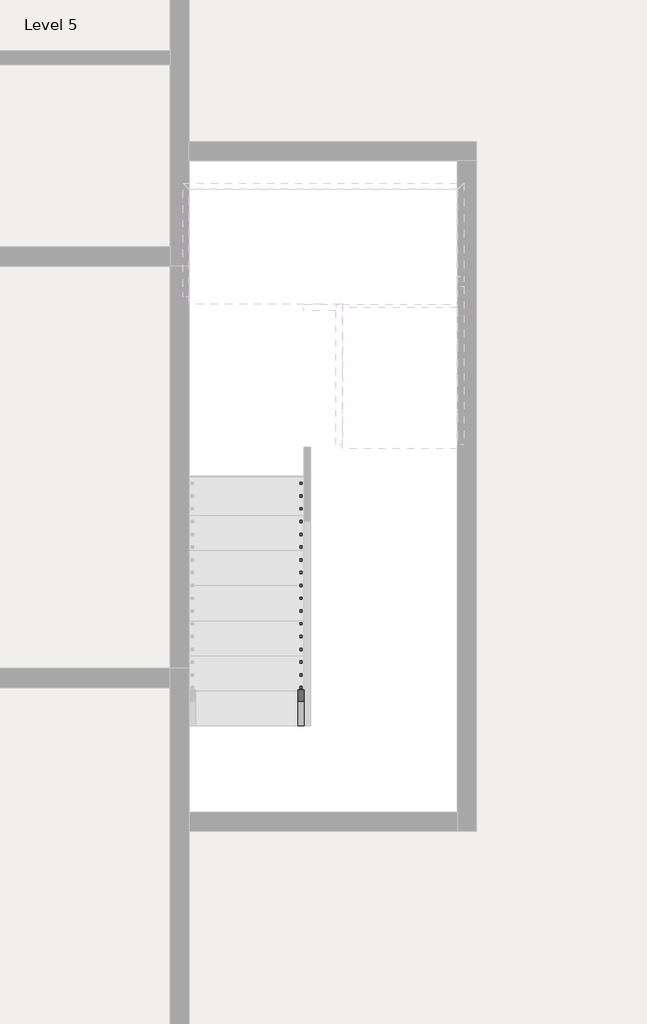
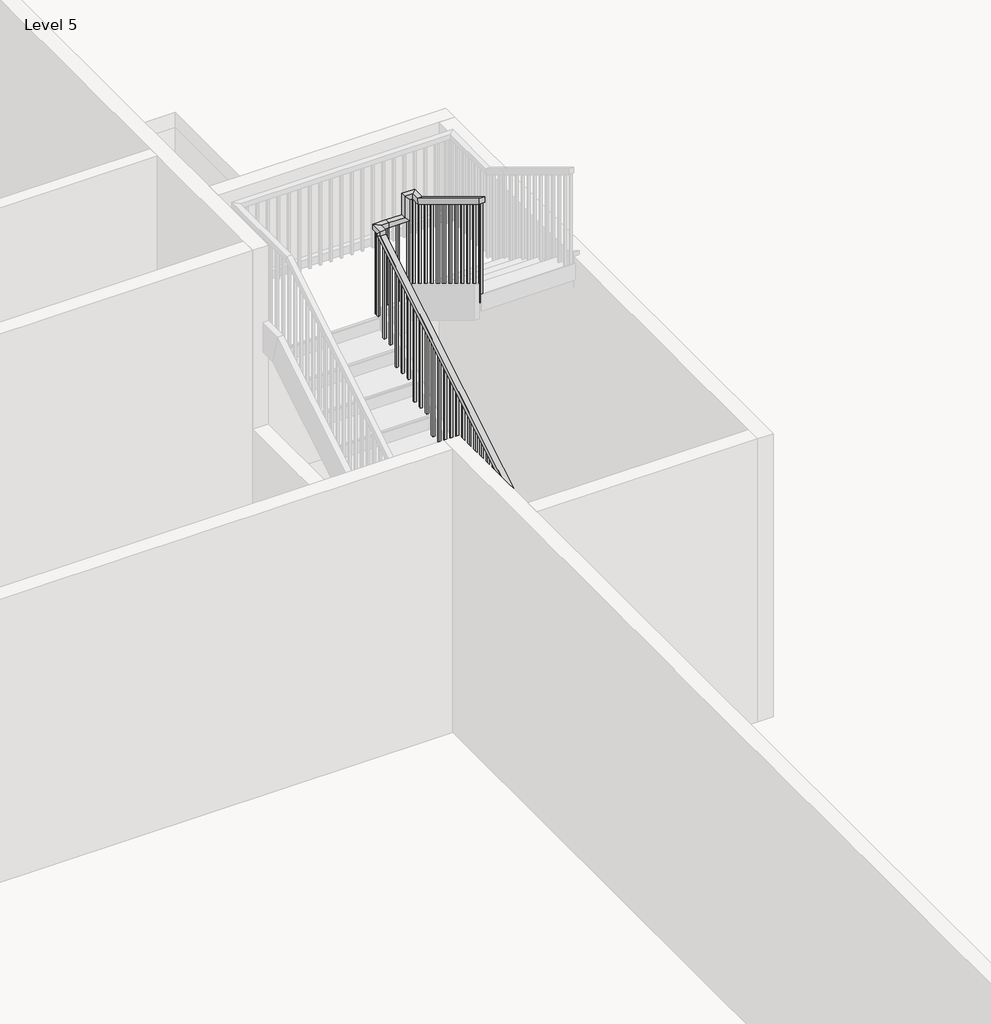
# One storey, part 7 of 8: 1 railing.
"""IFC4 building model written with IfcOpenShell, lengths in millimetres."""

from ifc_helpers import new_model, si_unit, frame, origin, place, context, project, spatial, polyline, outline, extrude, faceted_brep, element, save

model = new_model("IFC4")

# Units and contexts
model_context = context("Model", 3, world=origin())
ifc_project = project(units=[si_unit("LENGTHUNIT", "METRE", prefix="MILLI")], contexts=[model_context])

# Site, building, storey
site = spatial("IfcSite", under=ifc_project)
building = spatial("IfcBuilding", under=site)
storey = spatial("IfcBuildingStorey", under=building, Name="Level 5", Elevation=37426.6172466)

# Railing
placement = place(None, origin())
element("IfcRailing", 1, ObjectType="Handrail - Rectangular", at=placement, inside=storey, context=model_context, shape_type="SolidModel", body=[
    faceted_brep([(-2753.8415084, 19841.9216096, 38510.3505799), (-2753.8415084, 19841.9216096, 38450.9491197), (-2703.0415084, 19841.9216096, 38450.9491197), (-2703.0415084, 19841.9216096, 38510.3505799), (-2753.8415084, 23118.5216096, 40496.1687618), (-2753.8415084, 23169.3216096, 40467.5551803), (-2703.0415084, 23169.3216096, 40467.5551803), (-2703.0415084, 23118.5216096, 40496.1687618), (-2753.8415084, 23118.5216096, 40542.3505799), (-2753.8415084, 23169.3216096, 40491.5505799), (-2703.0415084, 23169.3216096, 40491.5505799), (-2703.0415084, 23118.5216096, 40542.3505799), (-2753.8415084, 23245.5216096, 40542.3505799), (-2753.8415084, 23245.5216096, 40491.5505799), (-2703.0415084, 23194.7216096, 40491.5505799), (-2703.0415084, 23194.7216096, 40542.3505799), (-2626.8415084, 23245.5216096, 40542.3505799), (-2626.8415084, 23245.5216096, 40491.5505799), (-2626.8415084, 23194.7216096, 40491.5505799), (-2626.8415084, 23194.7216096, 40542.3505799), (-2474.4415084, 23245.5216096, 40542.3505799), (-2423.6415084, 23245.5216096, 40491.5505799), (-2423.6415084, 23194.7216096, 40491.5505799), (-2474.4415084, 23194.7216096, 40542.3505799), (-2474.4415084, 23245.5216096, 40757.8657314), (-2423.6415084, 23245.5216096, 40707.0657314), (-2423.6415084, 23194.7216096, 40707.0657314), (-2474.4415084, 23194.7216096, 40757.8657314), (-2347.4415084, 23245.5216096, 40757.8657314), (-2347.4415084, 23245.5216096, 40707.0657314), (-2398.2415084, 23194.7216096, 40707.0657314), (-2398.2415084, 23194.7216096, 40757.8657314), (-2347.4415084, 23118.5216096, 40757.8657314), (-2347.4415084, 23104.3292002, 40707.0657314), (-2398.2415084, 23104.3292002, 40707.0657314), (-2398.2415084, 23118.5216096, 40757.8657314), (-2347.4415084, 22077.1216096, 41389.0172466), (-2398.2415084, 22077.1216096, 41389.0172466), (-2398.2415084, 22077.1216096, 41329.6157863), (-2347.4415084, 22077.1216096, 41329.6157863)], [[[0, 1, 2, 3]], [[1, 0, 4, 5]], [[2, 1, 5, 6]], [[3, 2, 6, 7]], [[0, 3, 7, 4]], [[5, 4, 8, 9]], [[6, 5, 9, 10]], [[7, 6, 10, 11]], [[4, 7, 11, 8]], [[9, 8, 12, 13]], [[10, 9, 13, 14]], [[11, 10, 14, 15]], [[8, 11, 15, 12]], [[13, 12, 16, 17]], [[14, 13, 17, 18]], [[15, 14, 18, 19]], [[12, 15, 19, 16]], [[17, 16, 20, 21]], [[18, 17, 21, 22]], [[19, 18, 22, 23]], [[16, 19, 23, 20]], [[21, 20, 24, 25]], [[22, 21, 25, 26]], [[23, 22, 26, 27]], [[20, 23, 27, 24]], [[25, 24, 28, 29]], [[26, 25, 29, 30]], [[27, 26, 30, 31]], [[24, 27, 31, 28]], [[29, 28, 32, 33]], [[30, 29, 33, 34]], [[31, 30, 34, 35]], [[28, 31, 35, 32]], [[36, 37, 38, 39]], [[33, 32, 36, 39]], [[34, 33, 39, 38]], [[35, 34, 38, 37]], [[32, 35, 37, 36]]]),
    extrude(outline(polyline([(22092.9966096, 41319.9945742), (22112.0466096, 41308.4491197), (22112.0466096, 40305.2839133), (22092.9966096, 40305.2839133), (22092.9966096, 41319.9945742)])), frame((-2382.3665084, 0.0, 0.0), z_axis=(1.0, 0.0, 0.0), x_axis=(0.0, 1.0, 0.0)), (0.0, 0.0, 1.0), 19.05),
    extrude(outline(polyline([(22194.5966096, 41258.4188166), (22213.6466096, 41246.8733621), (22213.6466096, 40305.2839133), (22194.5966096, 40305.2839133), (22194.5966096, 41258.4188166)])), frame((-2382.3665084, 0.0, 0.0), z_axis=(1.0, 0.0, 0.0), x_axis=(0.0, 1.0, 0.0)), (0.0, 0.0, 1.0), 19.05),
    extrude(outline(polyline([(22296.1966096, 41196.8430591), (22315.2466096, 41185.2976045), (22315.2466096, 40305.2839133), (22296.1966096, 40305.2839133), (22296.1966096, 41196.8430591)])), frame((-2382.3665084, 0.0, 0.0), z_axis=(1.0, 0.0, 0.0), x_axis=(0.0, 1.0, 0.0)), (0.0, 0.0, 1.0), 19.05),
    extrude(outline(polyline([(22397.7966096, 41135.2673015), (22416.8466096, 41123.721847), (22416.8466096, 40135.9505799), (22397.7966096, 40135.9505799), (22397.7966096, 41135.2673015)])), frame((-2382.3665084, 0.0, 0.0), z_axis=(1.0, 0.0, 0.0), x_axis=(0.0, 1.0, 0.0)), (0.0, 0.0, 1.0), 19.05),
    extrude(outline(polyline([(22499.3966096, 41073.6915439), (22518.4466096, 41062.1460894), (22518.4466096, 40135.9505799), (22499.3966096, 40135.9505799), (22499.3966096, 41073.6915439)])), frame((-2382.3665084, 0.0, 0.0), z_axis=(1.0, 0.0, 0.0), x_axis=(0.0, 1.0, 0.0)), (0.0, 0.0, 1.0), 19.05),
    extrude(outline(polyline([(22600.9966096, 41012.1157863), (22620.0466096, 41000.5703318), (22620.0466096, 40135.9505799), (22600.9966096, 40135.9505799), (22600.9966096, 41012.1157863)])), frame((-2382.3665084, 0.0, 0.0), z_axis=(1.0, 0.0, 0.0), x_axis=(0.0, 1.0, 0.0)), (0.0, 0.0, 1.0), 19.05),
    extrude(outline(polyline([(22702.5966096, 40950.5400288), (22721.6466096, 40938.9945742), (22721.6466096, 39966.6172466), (22702.5966096, 39966.6172466), (22702.5966096, 40950.5400288)])), frame((-2382.3665084, 0.0, 0.0), z_axis=(1.0, 0.0, 0.0), x_axis=(0.0, 1.0, 0.0)), (0.0, 0.0, 1.0), 19.05),
    extrude(outline(polyline([(22804.1966096, 40888.9642712), (22823.2466096, 40877.4188166), (22823.2466096, 39966.6172466), (22804.1966096, 39966.6172466), (22804.1966096, 40888.9642712)])), frame((-2382.3665084, 0.0, 0.0), z_axis=(1.0, 0.0, 0.0), x_axis=(0.0, 1.0, 0.0)), (0.0, 0.0, 1.0), 19.05),
    extrude(outline(polyline([(22905.7966096, 40827.3885136), (22924.8466096, 40815.8430591), (22924.8466096, 39966.6172466), (22905.7966096, 39966.6172466), (22905.7966096, 40827.3885136)])), frame((-2382.3665084, 0.0, 0.0), z_axis=(1.0, 0.0, 0.0), x_axis=(0.0, 1.0, 0.0)), (0.0, 0.0, 1.0), 19.05),
    extrude(outline(polyline([(23007.3966096, 40765.812756), (23026.4466096, 40754.2673015), (23026.4466096, 39797.2839133), (23007.3966096, 39797.2839133), (23007.3966096, 40765.812756)])), frame((-2382.3665084, 0.0, 0.0), z_axis=(1.0, 0.0, 0.0), x_axis=(0.0, 1.0, 0.0)), (0.0, 0.0, 1.0), 19.05),
    extrude(outline(polyline([(23108.9966096, 40704.2369985), (23128.0466096, 40692.6915439), (23128.0466096, 39797.2839133), (23108.9966096, 39797.2839133), (23108.9966096, 40704.2369985)])), frame((-2382.3665084, 0.0, 0.0), z_axis=(1.0, 0.0, 0.0), x_axis=(0.0, 1.0, 0.0)), (0.0, 0.0, 1.0), 19.05),
    extrude(outline(polyline([(-2433.1665084, 23210.5966096), (-2433.1665084, 23229.6466096), (-2414.1165084, 23229.6466096), (-2414.1165084, 23210.5966096), (-2433.1665084, 23210.5966096)])), frame((0.0, 0.0, 39627.9505799), z_axis=(0.0, 0.0, 1.0), x_axis=(1.0, 0.0, 0.0)), (0.0, 0.0, 1.0), 1079.1151515),
    extrude(outline(polyline([(-2534.7665084, 23210.5966096), (-2534.7665084, 23229.6466096), (-2515.7165084, 23229.6466096), (-2515.7165084, 23210.5966096), (-2534.7665084, 23210.5966096)])), frame((0.0, 0.0, 39627.9505799), z_axis=(0.0, 0.0, 1.0), x_axis=(1.0, 0.0, 0.0)), (0.0, 0.0, 1.0), 863.6),
    extrude(outline(polyline([(-2636.3665084, 23210.5966096), (-2636.3665084, 23229.6466096), (-2617.3165084, 23229.6466096), (-2617.3165084, 23210.5966096), (-2636.3665084, 23210.5966096)])), frame((0.0, 0.0, 39627.9505799), z_axis=(0.0, 0.0, 1.0), x_axis=(1.0, 0.0, 0.0)), (0.0, 0.0, 1.0), 863.6),
    extrude(outline(polyline([(-2718.9165084, 23185.1966096), (-2737.9665084, 23185.1966096), (-2737.9665084, 23204.2466096), (-2718.9165084, 23204.2466096), (-2718.9165084, 23185.1966096)])), frame((0.0, 0.0, 39627.9505799), z_axis=(0.0, 0.0, 1.0), x_axis=(1.0, 0.0, 0.0)), (0.0, 0.0, 1.0), 863.6),
    extrude(outline(polyline([(23083.5966096, 40415.6006348), (23102.6466096, 40427.1460894), (23102.6466096, 39458.6172466), (23083.5966096, 39458.6172466), (23083.5966096, 40415.6006348)])), frame((-2737.9665084, 0.0, 0.0), z_axis=(1.0, 0.0, 0.0), x_axis=(0.0, 1.0, 0.0)), (0.0, 0.0, 1.0), 19.05),
    extrude(outline(polyline([(22981.9966096, 40354.0248773), (23001.0466096, 40365.5703318), (23001.0466096, 39458.6172466), (22981.9966096, 39458.6172466), (22981.9966096, 40354.0248773)])), frame((-2737.9665084, 0.0, 0.0), z_axis=(1.0, 0.0, 0.0), x_axis=(0.0, 1.0, 0.0)), (0.0, 0.0, 1.0), 19.05),
    extrude(outline(polyline([(22880.3966096, 40292.4491197), (22899.4466096, 40303.9945742), (22899.4466096, 39289.2839133), (22880.3966096, 39289.2839133), (22880.3966096, 40292.4491197)])), frame((-2737.9665084, 0.0, 0.0), z_axis=(1.0, 0.0, 0.0), x_axis=(0.0, 1.0, 0.0)), (0.0, 0.0, 1.0), 19.05),
    extrude(outline(polyline([(22778.7966096, 40230.8733621), (22797.8466096, 40242.4188166), (22797.8466096, 39289.2839133), (22778.7966096, 39289.2839133), (22778.7966096, 40230.8733621)])), frame((-2737.9665084, 0.0, 0.0), z_axis=(1.0, 0.0, 0.0), x_axis=(0.0, 1.0, 0.0)), (0.0, 0.0, 1.0), 19.05),
    extrude(outline(polyline([(22677.1966096, 40169.2976045), (22696.2466096, 40180.8430591), (22696.2466096, 39289.2839133), (22677.1966096, 39289.2839133), (22677.1966096, 40169.2976045)])), frame((-2737.9665084, 0.0, 0.0), z_axis=(1.0, 0.0, 0.0), x_axis=(0.0, 1.0, 0.0)), (0.0, 0.0, 1.0), 19.05),
    extrude(outline(polyline([(22575.5966096, 40107.721847), (22594.6466096, 40119.2673015), (22594.6466096, 39119.9505799), (22575.5966096, 39119.9505799), (22575.5966096, 40107.721847)])), frame((-2737.9665084, 0.0, 0.0), z_axis=(1.0, 0.0, 0.0), x_axis=(0.0, 1.0, 0.0)), (0.0, 0.0, 1.0), 19.05),
    extrude(outline(polyline([(22473.9966096, 40046.1460894), (22493.0466096, 40057.6915439), (22493.0466096, 39119.9505799), (22473.9966096, 39119.9505799), (22473.9966096, 40046.1460894)])), frame((-2737.9665084, 0.0, 0.0), z_axis=(1.0, 0.0, 0.0), x_axis=(0.0, 1.0, 0.0)), (0.0, 0.0, 1.0), 19.05),
    extrude(outline(polyline([(22372.3966096, 39984.5703318), (22391.4466096, 39996.1157863), (22391.4466096, 39119.9505799), (22372.3966096, 39119.9505799), (22372.3966096, 39984.5703318)])), frame((-2737.9665084, 0.0, 0.0), z_axis=(1.0, 0.0, 0.0), x_axis=(0.0, 1.0, 0.0)), (0.0, 0.0, 1.0), 19.05),
    extrude(outline(polyline([(22270.7966096, 39922.9945742), (22289.8466096, 39934.5400288), (22289.8466096, 38950.6172466), (22270.7966096, 38950.6172466), (22270.7966096, 39922.9945742)])), frame((-2737.9665084, 0.0, 0.0), z_axis=(1.0, 0.0, 0.0), x_axis=(0.0, 1.0, 0.0)), (0.0, 0.0, 1.0), 19.05),
    extrude(outline(polyline([(22169.1966096, 39861.4188166), (22188.2466096, 39872.9642712), (22188.2466096, 38950.6172466), (22169.1966096, 38950.6172466), (22169.1966096, 39861.4188166)])), frame((-2737.9665084, 0.0, 0.0), z_axis=(1.0, 0.0, 0.0), x_axis=(0.0, 1.0, 0.0)), (0.0, 0.0, 1.0), 19.05),
    extrude(outline(polyline([(22067.5966096, 39799.8430591), (22086.6466096, 39811.3885136), (22086.6466096, 38950.6172466), (22067.5966096, 38950.6172466), (22067.5966096, 39799.8430591)])), frame((-2737.9665084, 0.0, 0.0), z_axis=(1.0, 0.0, 0.0), x_axis=(0.0, 1.0, 0.0)), (0.0, 0.0, 1.0), 19.05),
    extrude(outline(polyline([(21965.9966096, 39738.2673015), (21985.0466096, 39749.812756), (21985.0466096, 38781.2839133), (21965.9966096, 38781.2839133), (21965.9966096, 39738.2673015)])), frame((-2737.9665084, 0.0, 0.0), z_axis=(1.0, 0.0, 0.0), x_axis=(0.0, 1.0, 0.0)), (0.0, 0.0, 1.0), 19.05),
    extrude(outline(polyline([(21864.3966096, 39676.6915439), (21883.4466096, 39688.2369985), (21883.4466096, 38781.2839133), (21864.3966096, 38781.2839133), (21864.3966096, 39676.6915439)])), frame((-2737.9665084, 0.0, 0.0), z_axis=(1.0, 0.0, 0.0), x_axis=(0.0, 1.0, 0.0)), (0.0, 0.0, 1.0), 19.05),
    extrude(outline(polyline([(21762.7966096, 39615.1157863), (21781.8466096, 39626.6612409), (21781.8466096, 38611.9505799), (21762.7966096, 38611.9505799), (21762.7966096, 39615.1157863)])), frame((-2737.9665084, 0.0, 0.0), z_axis=(1.0, 0.0, 0.0), x_axis=(0.0, 1.0, 0.0)), (0.0, 0.0, 1.0), 19.05),
    extrude(outline(polyline([(21661.1966096, 39553.5400288), (21680.2466096, 39565.0854833), (21680.2466096, 38611.9505799), (21661.1966096, 38611.9505799), (21661.1966096, 39553.5400288)])), frame((-2737.9665084, 0.0, 0.0), z_axis=(1.0, 0.0, 0.0), x_axis=(0.0, 1.0, 0.0)), (0.0, 0.0, 1.0), 19.05),
    extrude(outline(polyline([(21559.5966096, 39491.9642712), (21578.6466096, 39503.5097257), (21578.6466096, 38611.9505799), (21559.5966096, 38611.9505799), (21559.5966096, 39491.9642712)])), frame((-2737.9665084, 0.0, 0.0), z_axis=(1.0, 0.0, 0.0), x_axis=(0.0, 1.0, 0.0)), (0.0, 0.0, 1.0), 19.05),
    extrude(outline(polyline([(21457.9966096, 39430.3885136), (21477.0466096, 39441.9339682), (21477.0466096, 38442.6172466), (21457.9966096, 38442.6172466), (21457.9966096, 39430.3885136)])), frame((-2737.9665084, 0.0, 0.0), z_axis=(1.0, 0.0, 0.0), x_axis=(0.0, 1.0, 0.0)), (0.0, 0.0, 1.0), 19.05),
    extrude(outline(polyline([(21356.3966096, 39368.812756), (21375.4466096, 39380.3582106), (21375.4466096, 38442.6172466), (21356.3966096, 38442.6172466), (21356.3966096, 39368.812756)])), frame((-2737.9665084, 0.0, 0.0), z_axis=(1.0, 0.0, 0.0), x_axis=(0.0, 1.0, 0.0)), (0.0, 0.0, 1.0), 19.05),
    extrude(outline(polyline([(21254.7966096, 39307.2369985), (21273.8466096, 39318.782453), (21273.8466096, 38442.6172466), (21254.7966096, 38442.6172466), (21254.7966096, 39307.2369985)])), frame((-2737.9665084, 0.0, 0.0), z_axis=(1.0, 0.0, 0.0), x_axis=(0.0, 1.0, 0.0)), (0.0, 0.0, 1.0), 19.05),
    extrude(outline(polyline([(21153.1966096, 39245.6612409), (21172.2466096, 39257.2066954), (21172.2466096, 38273.2839133), (21153.1966096, 38273.2839133), (21153.1966096, 39245.6612409)])), frame((-2737.9665084, 0.0, 0.0), z_axis=(1.0, 0.0, 0.0), x_axis=(0.0, 1.0, 0.0)), (0.0, 0.0, 1.0), 19.05),
    extrude(outline(polyline([(21051.5966096, 39184.0854833), (21070.6466096, 39195.6309379), (21070.6466096, 38273.2839133), (21051.5966096, 38273.2839133), (21051.5966096, 39184.0854833)])), frame((-2737.9665084, 0.0, 0.0), z_axis=(1.0, 0.0, 0.0), x_axis=(0.0, 1.0, 0.0)), (0.0, 0.0, 1.0), 19.05),
    extrude(outline(polyline([(20949.9966096, 39122.5097257), (20969.0466096, 39134.0551803), (20969.0466096, 38273.2839133), (20949.9966096, 38273.2839133), (20949.9966096, 39122.5097257)])), frame((-2737.9665084, 0.0, 0.0), z_axis=(1.0, 0.0, 0.0), x_axis=(0.0, 1.0, 0.0)), (0.0, 0.0, 1.0), 19.05),
    extrude(outline(polyline([(20848.3966096, 39060.9339682), (20867.4466096, 39072.4794227), (20867.4466096, 38103.9505799), (20848.3966096, 38103.9505799), (20848.3966096, 39060.9339682)])), frame((-2737.9665084, 0.0, 0.0), z_axis=(1.0, 0.0, 0.0), x_axis=(0.0, 1.0, 0.0)), (0.0, 0.0, 1.0), 19.05),
    extrude(outline(polyline([(20746.7966096, 38999.3582106), (20765.8466096, 39010.9036651), (20765.8466096, 38103.9505799), (20746.7966096, 38103.9505799), (20746.7966096, 38999.3582106)])), frame((-2737.9665084, 0.0, 0.0), z_axis=(1.0, 0.0, 0.0), x_axis=(0.0, 1.0, 0.0)), (0.0, 0.0, 1.0), 19.05),
    extrude(outline(polyline([(20645.1966096, 38937.782453), (20664.2466096, 38949.3279076), (20664.2466096, 37934.6172466), (20645.1966096, 37934.6172466), (20645.1966096, 38937.782453)])), frame((-2737.9665084, 0.0, 0.0), z_axis=(1.0, 0.0, 0.0), x_axis=(0.0, 1.0, 0.0)), (0.0, 0.0, 1.0), 19.05),
    extrude(outline(polyline([(20543.5966096, 38876.2066954), (20562.6466096, 38887.75215), (20562.6466096, 37934.6172466), (20543.5966096, 37934.6172466), (20543.5966096, 38876.2066954)])), frame((-2737.9665084, 0.0, 0.0), z_axis=(1.0, 0.0, 0.0), x_axis=(0.0, 1.0, 0.0)), (0.0, 0.0, 1.0), 19.05),
    extrude(outline(polyline([(20441.9966096, 38814.6309379), (20461.0466096, 38826.1763924), (20461.0466096, 37934.6172466), (20441.9966096, 37934.6172466), (20441.9966096, 38814.6309379)])), frame((-2737.9665084, 0.0, 0.0), z_axis=(1.0, 0.0, 0.0), x_axis=(0.0, 1.0, 0.0)), (0.0, 0.0, 1.0), 19.05),
    extrude(outline(polyline([(20340.3966096, 38753.0551803), (20359.4466096, 38764.6006348), (20359.4466096, 37765.2839133), (20340.3966096, 37765.2839133), (20340.3966096, 38753.0551803)])), frame((-2737.9665084, 0.0, 0.0), z_axis=(1.0, 0.0, 0.0), x_axis=(0.0, 1.0, 0.0)), (0.0, 0.0, 1.0), 19.05),
    extrude(outline(polyline([(20238.7966096, 38691.4794227), (20257.8466096, 38703.0248773), (20257.8466096, 37765.2839133), (20238.7966096, 37765.2839133), (20238.7966096, 38691.4794227)])), frame((-2737.9665084, 0.0, 0.0), z_axis=(1.0, 0.0, 0.0), x_axis=(0.0, 1.0, 0.0)), (0.0, 0.0, 1.0), 19.05),
    extrude(outline(polyline([(20137.1966096, 38629.9036651), (20156.2466096, 38641.4491197), (20156.2466096, 37765.2839133), (20137.1966096, 37765.2839133), (20137.1966096, 38629.9036651)])), frame((-2737.9665084, 0.0, 0.0), z_axis=(1.0, 0.0, 0.0), x_axis=(0.0, 1.0, 0.0)), (0.0, 0.0, 1.0), 19.05),
    extrude(outline(polyline([(20035.5966096, 38568.3279076), (20054.6466096, 38579.8733621), (20054.6466096, 37595.9505799), (20035.5966096, 37595.9505799), (20035.5966096, 38568.3279076)])), frame((-2737.9665084, 0.0, 0.0), z_axis=(1.0, 0.0, 0.0), x_axis=(0.0, 1.0, 0.0)), (0.0, 0.0, 1.0), 19.05),
    extrude(outline(polyline([(19933.9966096, 38506.75215), (19953.0466096, 38518.2976045), (19953.0466096, 37595.9505799), (19933.9966096, 37595.9505799), (19933.9966096, 38506.75215)])), frame((-2737.9665084, 0.0, 0.0), z_axis=(1.0, 0.0, 0.0), x_axis=(0.0, 1.0, 0.0)), (0.0, 0.0, 1.0), 19.05),
    extrude(outline(polyline([(-2382.3665084, 23210.5966096), (-2382.3665084, 23229.6466096), (-2363.3165084, 23229.6466096), (-2363.3165084, 23210.5966096), (-2382.3665084, 23210.5966096)])), frame((0.0, 0.0, 39627.9505799), z_axis=(0.0, 0.0, 1.0), x_axis=(1.0, 0.0, 0.0)), (0.0, 0.0, 1.0), 1079.1151515),
    extrude(outline(polyline([(-2718.9165084, 23210.5966096), (-2737.9665084, 23210.5966096), (-2737.9665084, 23229.6466096), (-2718.9165084, 23229.6466096), (-2718.9165084, 23210.5966096)])), frame((0.0, 0.0, 39627.9505799), z_axis=(0.0, 0.0, 1.0), x_axis=(1.0, 0.0, 0.0)), (0.0, 0.0, 1.0), 863.6),
    extrude(outline(polyline([(22077.1216096, 41329.6157863), (22096.1716096, 41318.0703318), (22096.1716096, 40305.2839133), (22077.1216096, 40305.2839133), (22077.1216096, 41329.6157863)])), frame((-2382.3665084, 0.0, 0.0), z_axis=(1.0, 0.0, 0.0), x_axis=(0.0, 1.0, 0.0)), (0.0, 0.0, 1.0), 19.05),
    extrude(outline(polyline([(19841.9216096, 38450.9491197), (19860.9716096, 38462.4945742), (19860.9716096, 37595.9505799), (19841.9216096, 37595.9505799), (19841.9216096, 38450.9491197)])), frame((-2737.9665084, 0.0, 0.0), z_axis=(1.0, 0.0, 0.0), x_axis=(0.0, 1.0, 0.0)), (0.0, 0.0, 1.0), 19.05),
])

save(model, "model.ifc")

# Revit data of these elements
# Type "Handrail - Rectangular"
#   Assembly Code = "C2010400"
#   built-in parameter 1008612 = 0.0416667 (stored number, unit not read)
#   built-in parameter 1008611 = 0.0416667 (stored number, unit not read)
#   built-in parameter 1008609 = 0.333333 (stored number, unit not read)
#   built-in parameter 1008604 = 0.166667 (stored number, unit not read)
#   built-in parameter 1008603 = 0.166667 (stored number, unit not read)
#   Railing Height = 3' - 0"
#   built-in parameter 1008630 = 2
#   built-in parameter 1008610 = 2
#   built-in parameter 1008618 = Baluster - Square : 3/4"
# Element 1 (IfcRailing, "Handrail - Rectangular")
#   Phase Created = New Construction
